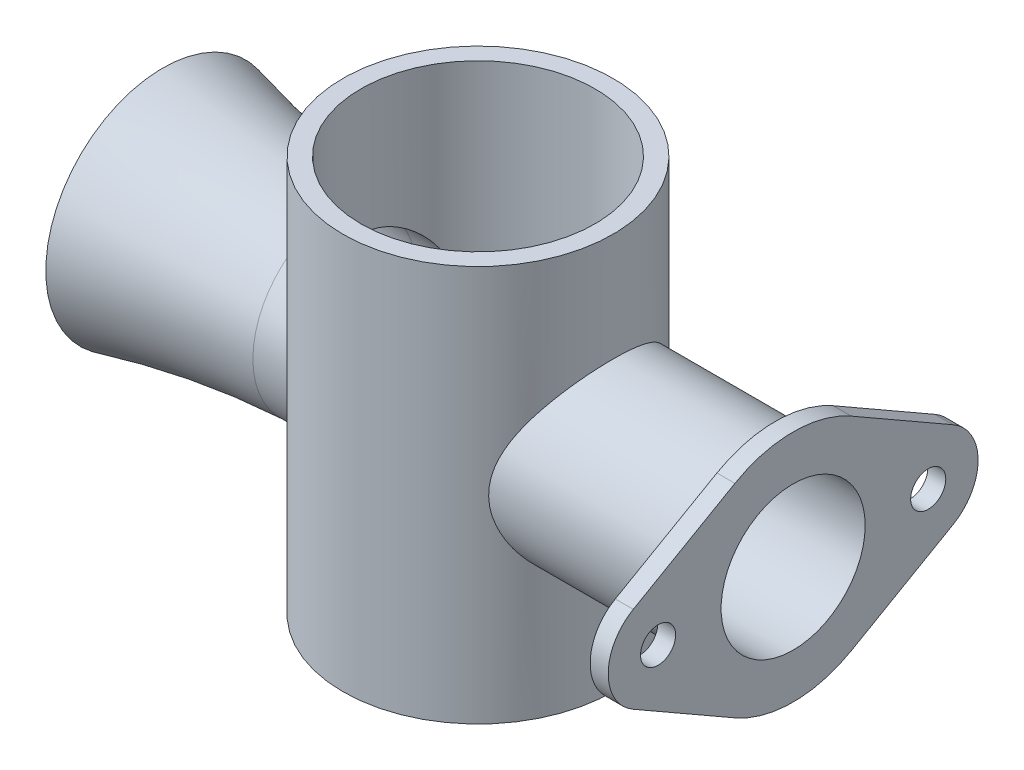
from build123d import *
from build123d.topology import SkipClean

# Parameters (mm, degrees)
MAIN_BARREL_SKETCH_R       = 7.5
MAIN_BARREL_DEPTH          = 11
MAIN_BORE_SKETCH_13_R      = 6.5
MAIN_BORE_13_DEPTH         = 20
OUTLET_TUBE_SKETCH_10_R    = 5
OUTLET_TUBE_10_DEPTH       = 9
MOUNTING_FLANGE_SKETCH_R   = 4
MOUNTING_FLANGE_SKETCH_R_2 = 0.975
MOUNTING_FLANGE_DEPTH      = 1
OUTLET_TUBE_JOINT_REACH    = 23.248
OUTLET_TUBE_JOINT_SKETCH_R = 5
INTAKE_TUBE_10_REACH       = 31.18
INTAKE_TUBE_SKETCH_10_R    = 5
OUTLET_BORE_SKETCH_R       = 4
OUTLET_BORE_DEPTH          = 38.181620489
SIDE_PORT_SKETCH_3_R       = 1.5
SIDE_PORT_3_DEPTH          = 2


with BuildPart() as part:
    # Main Barrel Sketch → Main Barrel (new, symmetric)
    with BuildSketch(Plane(origin=(0, 0, 0), x_dir=(1, 0, 0), z_dir=(0, 1, 0))):
        with Locations(Location((0, 0, 0), (0, 0, 270))):
            Circle(MAIN_BARREL_SKETCH_R)
    extrude(amount=MAIN_BARREL_DEPTH, both=True)

    # Main Bore Sketch Ø13 → Main Bore Ø13 (cut)
    with BuildSketch(Plane(origin=(0, 11, 0), x_dir=(1, 0, 0), z_dir=(0, 1, 0))):
        with Locations(Location((0, 0, 0), (0, 0, 270))):
            Circle(MAIN_BORE_SKETCH_13_R)
    extrude(amount=-MAIN_BORE_13_DEPTH, mode=Mode.SUBTRACT)

    # Outlet Tube Joint Sketch → Outlet Tube Joint (add, up to next)
    with BuildSketch(Plane.ZY.offset(-7.5), mode=Mode.PRIVATE) as outlet_tube_joint_sk1:
        with Locations(Location((0, 0, 0), (0, 0, 180))):
            Circle(OUTLET_TUBE_JOINT_SKETCH_R)
    outlet_tube_joint_tool1 = extrude(outlet_tube_joint_sk1.sketch, amount=OUTLET_TUBE_JOINT_REACH, mode=Mode.PRIVATE) - part.part


with BuildPart() as body_2:
    # Outlet Tube Sketch Ø10 → Outlet Tube Ø10 (new body)
    with BuildSketch(Plane.ZY.offset(-7.5)):
        Circle(OUTLET_TUBE_SKETCH_10_R)
    extrude(amount=-OUTLET_TUBE_10_DEPTH)

    # Mounting Flange Sketch → Mounting Flange (add)
    with BuildSketch(Plane(origin=(16.5, 0, 0), x_dir=(0, 0, -1), z_dir=(1, 0, 0))):
        with BuildLine():
            Line((3.232666667, 5.63913701), (8.877613333, 2.403139926))
            ThreePointArc((8.877613333, 2.403139926), (10.27, 0), (8.877613333, -2.403139926))
            Line((8.877613333, -2.403139926), (3.232666667, -5.63913701))
            ThreePointArc((3.232666667, -5.63913701), (0, -6.5), (-3.232666667, -5.63913701))
            Line((-3.232666667, -5.63913701), (-8.877613333, -2.403139926))
            ThreePointArc((-8.877613333, -2.403139926), (-10.27, 0), (-8.877613333, 2.403139926))
            Line((-8.877613333, 2.403139926), (-3.232666667, 5.63913701))
            ThreePointArc((-3.232666667, 5.63913701), (0, 6.5), (3.232666667, 5.63913701))
        make_face()
        Circle(MOUNTING_FLANGE_SKETCH_R, mode=Mode.SUBTRACT)
        with Locations((7.5, 0)):
            Circle(MOUNTING_FLANGE_SKETCH_R_2, mode=Mode.SUBTRACT)
        with Locations(Location((-7.5, 0, 0), (0, 0, 180))):
            Circle(MOUNTING_FLANGE_SKETCH_R_2, mode=Mode.SUBTRACT)
    extrude(amount=MOUNTING_FLANGE_DEPTH)


with BuildPart() as part_1:
    add(part.part)

    add(body_2.part)  # Outlet Tube Joint merges body 2
    add(outlet_tube_joint_tool1.solids().sort_by_distance((7.5, 0, 0))[0])
    add(outlet_tube_joint_tool1.solids().sort_by_distance((7.5, 0, 0))[1])

    # Intake Tube Sketch Ø10 → Intake Tube Ø10 (add, up to next)
    with BuildSketch(Plane(origin=(-7.5, 0, 0), x_dir=(0, 0, -1), z_dir=(1, 0, 0)), mode=Mode.PRIVATE) as intake_tube_10_sk1:
        Circle(INTAKE_TUBE_SKETCH_10_R)
    intake_tube_10_tool1 = extrude(intake_tube_10_sk1.sketch, amount=INTAKE_TUBE_10_REACH, mode=Mode.PRIVATE) - part_1.part


with BuildPart() as body_2_2:
    # Intake Bell Profile → Intake Bell (revolve)
    with BuildSketch(Plane.XY, mode=Mode.PRIVATE) as intake_bell_sk:
        with BuildLine():
            Line((-17.5, 6.5), (-17.5, 6))
            ThreePointArc((-17.5, 6), (-12.599019514, 4.504902432), (-7.5, 4))
            Line((-7.5, 4), (-7.5, 5))
            ThreePointArc((-7.5, 5), (-12.537638643, 5.499075714), (-17.5, 6.5))
        make_face()
    revolve(intake_bell_sk.sketch.rotate(Axis((0, 0, 0), (-1, 0, 0)), 90), axis=Axis((0, 0, 0), (-1, 0, 0)))


with BuildPart() as part_2:
    add(part_1.part)

    add(body_2_2.part)  # Intake Tube Ø10 merges body 2 2
    add(intake_tube_10_tool1.solids().sort_by_distance((-7.5, 0, 0))[0])
    add(intake_tube_10_tool1.solids().sort_by_distance((-7.5, 0, 0))[1])

    # Outlet Bore Sketch → Outlet Bore (cut, through all)
    with SkipClean():  # the faces are left unmerged after this step: merging them gives an invalid solid
        with BuildSketch(Plane(origin=(16.5, 0, 0), x_dir=(0, 0, -1), z_dir=(1, 0, 0))):
            Circle(OUTLET_BORE_SKETCH_R)
        extrude(amount=-OUTLET_BORE_DEPTH, mode=Mode.SUBTRACT)

    # Side Port Sketch Ø3 → Side Port Ø3 (cut)
    with SkipClean():  # the faces are left unmerged after this step: merging them gives an invalid solid
        with BuildSketch(Plane.XZ.offset(11)):
            with Locations(Location((0, 0, 0), (0, 0, 270))):
                Circle(SIDE_PORT_SKETCH_3_R)
        extrude(amount=-SIDE_PORT_3_DEPTH, mode=Mode.SUBTRACT)


solid = part_2.part
